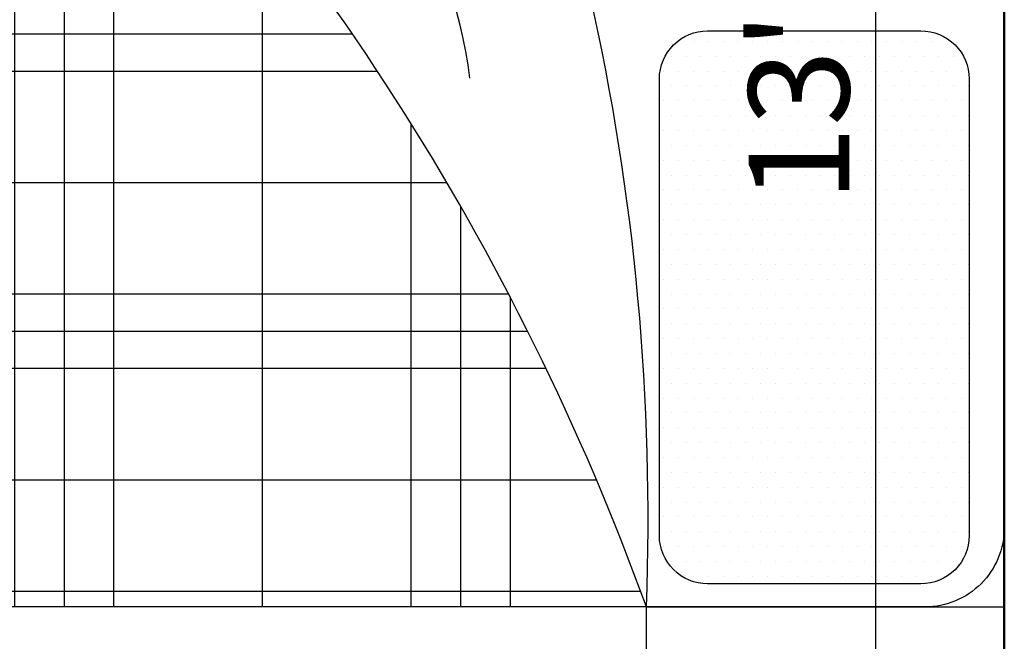
# Model space of a CAD drawing. Units: inches. Extents: x 3064 to 19385, y 846 to 15425.
# Tile 96 of 108: x 7612 to 7661, y 1032 to 1063. Entities that reach past the tile are written whole.
import ezdxf

# ---------------------------------------------------------------- set-up
doc = ezdxf.new("R2010")
doc.units = ezdxf.units.IN
for name, color, linetype, lineweight in [('A-ANNO-DIMS', 2, 'Continuous', 18), ('A-FLOR-FIXT', 9, 'Continuous', 18), ('A-WALL', 7, 'Continuous', 50)]:
    doc.layers.add(name, color=color, linetype=linetype, lineweight=lineweight)
doc.layers.add('BLOCK', color=6, linetype='Continuous')
doc.styles.get("Standard").update_dxf_attribs({"font": 'arial.ttf'})
doc.dimstyles.new('ISO-25', dxfattribs={"dimtxt": 9, "dimasz": 2.5, "dimexe": 1.25, "dimexo": 0.625, "dimtad": 1, "dimdec": 1, "dimlunit": 3, "dimtxsty": 'Standard', "dimcen": 2.5, "dimadec": 0, "dimazin": 0, "dimtfac": 1, "dimtdec": 1, "dimtmove": 0, "dimatfit": 3, "dimfxl": 1, "dimarcsym": 0})

# ---------------------------------------------------------------- blocks, each defined once
blk = doc.blocks.new('*D234')
at = {"layer": 'A-ANNO-DIMS', "color": 0, "lineweight": -2, "transparency": 16777216}
for p, q in [((7660.621, 1144.34), (7653.626, 1144.34)), ((7654.876, 984.84), (7654.876, 1141.84)), ((7660.621, 982.34), (7653.626, 982.34))]:
    blk.add_line(p, q, dxfattribs=at)
at = {"layer": 'A-ANNO-DIMS', "color": 0, "transparency": 16777216}
for points in [[(7654.459, 1141.84), (7655.292, 1141.84), (7654.876, 1144.34)], [(7654.459, 984.84), (7655.292, 984.84), (7654.876, 982.34)]]:
    blk.add_solid(points, dxfattribs=at)
at = {"layer": 'Defpoints', "color": 0, "transparency": 16777216}
for p in [(7654.876, 1144.34), (7661.246, 1144.34), (7661.246, 982.34)]:
    blk.add_point(p, dxfattribs=at)
at = {"layer": 'A-ANNO-DIMS', "color": 0, "transparency": 16777216, "insert": (7651.696, 1063.34), "char_height": 5, "attachment_point": 5, "rotation": 90}
blk.add_mtext('13\'-6"', dxfattribs=at)
blk = doc.blocks.new('*X5')
at = {"color": 0}
for p, q in [((276.598, 451.25), (280.51, 451.25)), ((275.455, 450.625), (280.51, 450.625)), ((274.411, 450), (280.51, 450)), ((265.51, 448.125), (267.634, 448.125)), ((271.723, 448.125), (280.51, 448.125)), ((265.51, 446.25), (268.465, 446.25)), ((269.519, 446.25), (280.51, 446.25)), ((265.51, 445.625), (268.531, 445.625)), ((268.866, 445.625), (280.51, 445.625)), ((265.51, 445), (280.51, 445)), ((265.51, 443.125), (280.51, 443.125)), ((265.51, 441.25), (280.51, 441.25)), ((265.51, 440.625), (280.51, 440.625)), ((265.634, 440), (280.386, 440))]:
    blk.add_line(p, q, dxfattribs=at)
blk = doc.blocks.new('*X6')
at = {"color": 0}
for p, q in [((280.312, 439.886), (280.312, 452.896)), ((278.906, 439.482), (278.906, 452.338)), ((277.5, 439.482), (277.5, 451.702)), ((277.031, 439.482), (277.031, 451.471)), ((276.562, 439.482), (276.562, 451.231)), ((275.156, 439.482), (275.156, 450.451)), ((273.75, 439.482), (273.75, 449.576)), ((273.281, 439.482), (273.281, 449.261))]:
    blk.add_line(p, q, dxfattribs=at)
blk = doc.blocks.new('*X7')
at = {"color": 0}
for p, q in [((273.9375, 457.03125), (273.9375, 457.03125)), ((274.3125, 457.03125), (274.3125, 457.03125)), ((274.6875, 457.03125), (274.6875, 457.03125)), ((275.0625, 457.03125), (275.0625, 457.03125)), ((275.4375, 457.03125), (275.4375, 457.03125)), ((275.8125, 457.03125), (275.8125, 457.03125)), ((276.1875, 457.03125), (276.1875, 457.03125)), ((276.5625, 457.03125), (276.5625, 457.03125)), ((276.9375, 457.03125), (276.9375, 457.03125)), ((277.3125, 457.03125), (277.3125, 457.03125)), ((277.6875, 457.03125), (277.6875, 457.03125)), ((278.0625, 457.03125), (278.0625, 457.03125)), ((278.4375, 457.03125), (278.4375, 457.03125)), ((278.8125, 457.03125), (278.8125, 457.03125)), ((279.1875, 457.03125), (279.1875, 457.03125)), ((279.5625, 457.03125), (279.5625, 457.03125)), ((273.75, 456.9375), (273.75, 456.9375)), ((274.125, 456.9375), (274.125, 456.9375)), ((274.5, 456.9375), (274.5, 456.9375)), ((274.875, 456.9375), (274.875, 456.9375)), ((275.25, 456.9375), (275.25, 456.9375)), ((275.625, 456.9375), (275.625, 456.9375)), ((276, 456.9375), (276, 456.9375)), ((276.375, 456.9375), (276.375, 456.9375)), ((276.75, 456.9375), (276.75, 456.9375)), ((277.125, 456.9375), (277.125, 456.9375)), ((277.5, 456.9375), (277.5, 456.9375)), ((277.875, 456.9375), (277.875, 456.9375)), ((278.25, 456.9375), (278.25, 456.9375)), ((278.625, 456.9375), (278.625, 456.9375)), ((279, 456.9375), (279, 456.9375)), ((279.375, 456.9375), (279.375, 456.9375)), ((279.75, 456.9375), (279.75, 456.9375)), ((273.5625, 456.84375), (273.5625, 456.84375)), ((273.9375, 456.84375), (273.9375, 456.84375)), ((274.3125, 456.84375), (274.3125, 456.84375)), ((274.6875, 456.84375), (274.6875, 456.84375)), ((275.0625, 456.84375), (275.0625, 456.84375)), ((275.4375, 456.84375), (275.4375, 456.84375)), ((275.8125, 456.84375), (275.8125, 456.84375)), ((276.1875, 456.84375), (276.1875, 456.84375)), ((276.5625, 456.84375), (276.5625, 456.84375)), ((276.9375, 456.84375), (276.9375, 456.84375)), ((277.3125, 456.84375), (277.3125, 456.84375)), ((277.6875, 456.84375), (277.6875, 456.84375)), ((278.0625, 456.84375), (278.0625, 456.84375)), ((278.4375, 456.84375), (278.4375, 456.84375)), ((278.8125, 456.84375), (278.8125, 456.84375)), ((279.1875, 456.84375), (279.1875, 456.84375)), ((279.5625, 456.84375), (279.5625, 456.84375)), ((279.9375, 456.84375), (279.9375, 456.84375)), ((273.375, 456.75), (273.375, 456.75)), ((273.5625, 456.65625), (273.5625, 456.65625)), ((273.75, 456.75), (273.75, 456.75)), ((273.9375, 456.65625), (273.9375, 456.65625)), ((274.125, 456.75), (274.125, 456.75)), ((274.3125, 456.65625), (274.3125, 456.65625)), ((274.5, 456.75), (274.5, 456.75)), ((274.6875, 456.65625), (274.6875, 456.65625)), ((274.875, 456.75), (274.875, 456.75)), ((275.0625, 456.65625), (275.0625, 456.65625)), ((275.25, 456.75), (275.25, 456.75)), ((275.4375, 456.65625), (275.4375, 456.65625)), ((275.625, 456.75), (275.625, 456.75)), ((275.8125, 456.65625), (275.8125, 456.65625)), ((276, 456.75), (276, 456.75)), ((276.1875, 456.65625), (276.1875, 456.65625)), ((276.375, 456.75), (276.375, 456.75)), ((276.5625, 456.65625), (276.5625, 456.65625)), ((276.75, 456.75), (276.75, 456.75)), ((276.9375, 456.65625), (276.9375, 456.65625)), ((277.125, 456.75), (277.125, 456.75)), ((277.3125, 456.65625), (277.3125, 456.65625)), ((277.5, 456.75), (277.5, 456.75)), ((277.6875, 456.65625), (277.6875, 456.65625)), ((277.875, 456.75), (277.875, 456.75)), ((278.0625, 456.65625), (278.0625, 456.65625)), ((278.25, 456.75), (278.25, 456.75)), ((278.4375, 456.65625), (278.4375, 456.65625)), ((278.625, 456.75), (278.625, 456.75)), ((278.8125, 456.65625), (278.8125, 456.65625)), ((279, 456.75), (279, 456.75)), ((279.1875, 456.65625), (279.1875, 456.65625)), ((279.375, 456.75), (279.375, 456.75)), ((279.5625, 456.65625), (279.5625, 456.65625)), ((279.75, 456.75), (279.75, 456.75)), ((279.9375, 456.65625), (279.9375, 456.65625)), ((280.125, 456.75), (280.125, 456.75)), ((273.375, 456.5625), (273.375, 456.5625)), ((273.75, 456.5625), (273.75, 456.5625)), ((274.125, 456.5625), (274.125, 456.5625)), ((274.5, 456.5625), (274.5, 456.5625)), ((274.875, 456.5625), (274.875, 456.5625)), ((275.25, 456.5625), (275.25, 456.5625)), ((275.625, 456.5625), (275.625, 456.5625)), ((276, 456.5625), (276, 456.5625)), ((276.375, 456.5625), (276.375, 456.5625)), ((276.75, 456.5625), (276.75, 456.5625)), ((277.125, 456.5625), (277.125, 456.5625)), ((277.5, 456.5625), (277.5, 456.5625)), ((277.875, 456.5625), (277.875, 456.5625)), ((278.25, 456.5625), (278.25, 456.5625)), ((278.625, 456.5625), (278.625, 456.5625)), ((279, 456.5625), (279, 456.5625)), ((279.375, 456.5625), (279.375, 456.5625)), ((279.75, 456.5625), (279.75, 456.5625)), ((280.125, 456.5625), (280.125, 456.5625)), ((273.5625, 456.46875), (273.5625, 456.46875)), ((273.9375, 456.46875), (273.9375, 456.46875)), ((274.3125, 456.46875), (274.3125, 456.46875)), ((274.6875, 456.46875), (274.6875, 456.46875)), ((275.0625, 456.46875), (275.0625, 456.46875)), ((275.4375, 456.46875), (275.4375, 456.46875)), ((275.8125, 456.46875), (275.8125, 456.46875)), ((276.1875, 456.46875), (276.1875, 456.46875)), ((276.5625, 456.46875), (276.5625, 456.46875)), ((276.9375, 456.46875), (276.9375, 456.46875)), ((277.3125, 456.46875), (277.3125, 456.46875)), ((277.6875, 456.46875), (277.6875, 456.46875)), ((278.0625, 456.46875), (278.0625, 456.46875)), ((278.4375, 456.46875), (278.4375, 456.46875)), ((278.8125, 456.46875), (278.8125, 456.46875)), ((279.1875, 456.46875), (279.1875, 456.46875)), ((279.5625, 456.46875), (279.5625, 456.46875)), ((279.9375, 456.46875), (279.9375, 456.46875)), ((273.375, 456.375), (273.375, 456.375)), ((273.75, 456.375), (273.75, 456.375)), ((274.125, 456.375), (274.125, 456.375)), ((274.5, 456.375), (274.5, 456.375)), ((274.875, 456.375), (274.875, 456.375)), ((275.25, 456.375), (275.25, 456.375)), ((275.625, 456.375), (275.625, 456.375)), ((276, 456.375), (276, 456.375)), ((276.375, 456.375), (276.375, 456.375)), ((276.75, 456.375), (276.75, 456.375)), ((277.125, 456.375), (277.125, 456.375)), ((277.5, 456.375), (277.5, 456.375)), ((277.875, 456.375), (277.875, 456.375)), ((278.25, 456.375), (278.25, 456.375)), ((278.625, 456.375), (278.625, 456.375)), ((279, 456.375), (279, 456.375)), ((279.375, 456.375), (279.375, 456.375)), ((279.75, 456.375), (279.75, 456.375)), ((280.125, 456.375), (280.125, 456.375)), ((273.375, 456.1875), (273.375, 456.1875)), ((273.5625, 456.28125), (273.5625, 456.28125)), ((273.75, 456.1875), (273.75, 456.1875)), ((273.9375, 456.28125), (273.9375, 456.28125)), ((274.125, 456.1875), (274.125, 456.1875)), ((274.3125, 456.28125), (274.3125, 456.28125)), ((274.5, 456.1875), (274.5, 456.1875)), ((274.6875, 456.28125), (274.6875, 456.28125)), ((274.875, 456.1875), (274.875, 456.1875)), ((275.0625, 456.28125), (275.0625, 456.28125)), ((275.25, 456.1875), (275.25, 456.1875)), ((275.4375, 456.28125), (275.4375, 456.28125)), ((275.625, 456.1875), (275.625, 456.1875)), ((275.8125, 456.28125), (275.8125, 456.28125)), ((276, 456.1875), (276, 456.1875)), ((276.1875, 456.28125), (276.1875, 456.28125)), ((276.375, 456.1875), (276.375, 456.1875)), ((276.5625, 456.28125), (276.5625, 456.28125)), ((276.75, 456.1875), (276.75, 456.1875)), ((276.9375, 456.28125), (276.9375, 456.28125)), ((277.125, 456.1875), (277.125, 456.1875)), ((277.3125, 456.28125), (277.3125, 456.28125)), ((277.5, 456.1875), (277.5, 456.1875)), ((277.6875, 456.28125), (277.6875, 456.28125)), ((277.875, 456.1875), (277.875, 456.1875)), ((278.0625, 456.28125), (278.0625, 456.28125)), ((278.25, 456.1875), (278.25, 456.1875)), ((278.4375, 456.28125), (278.4375, 456.28125)), ((278.625, 456.1875), (278.625, 456.1875)), ((278.8125, 456.28125), (278.8125, 456.28125)), ((279, 456.1875), (279, 456.1875)), ((279.1875, 456.28125), (279.1875, 456.28125)), ((279.375, 456.1875), (279.375, 456.1875)), ((279.5625, 456.28125), (279.5625, 456.28125)), ((279.75, 456.1875), (279.75, 456.1875)), ((279.9375, 456.28125), (279.9375, 456.28125)), ((280.125, 456.1875), (280.125, 456.1875)), ((273.5625, 456.09375), (273.5625, 456.09375)), ((273.9375, 456.09375), (273.9375, 456.09375)), ((274.3125, 456.09375), (274.3125, 456.09375)), ((274.6875, 456.09375), (274.6875, 456.09375)), ((275.0625, 456.09375), (275.0625, 456.09375)), ((275.4375, 456.09375), (275.4375, 456.09375)), ((275.8125, 456.09375), (275.8125, 456.09375)), ((276.1875, 456.09375), (276.1875, 456.09375)), ((276.5625, 456.09375), (276.5625, 456.09375)), ((276.9375, 456.09375), (276.9375, 456.09375)), ((277.3125, 456.09375), (277.3125, 456.09375)), ((277.6875, 456.09375), (277.6875, 456.09375)), ((278.0625, 456.09375), (278.0625, 456.09375)), ((278.4375, 456.09375), (278.4375, 456.09375)), ((278.8125, 456.09375), (278.8125, 456.09375)), ((279.1875, 456.09375), (279.1875, 456.09375)), ((279.5625, 456.09375), (279.5625, 456.09375)), ((279.9375, 456.09375), (279.9375, 456.09375)), ((273.375, 456), (273.375, 456)), ((273.75, 456), (273.75, 456)), ((274.125, 456), (274.125, 456)), ((274.5, 456), (274.5, 456)), ((274.875, 456), (274.875, 456)), ((275.25, 456), (275.25, 456)), ((275.625, 456), (275.625, 456)), ((276, 456), (276, 456)), ((276.375, 456), (276.375, 456)), ((276.75, 456), (276.75, 456)), ((277.125, 456), (277.125, 456)), ((277.5, 456), (277.5, 456)), ((277.875, 456), (277.875, 456)), ((278.25, 456), (278.25, 456)), ((278.625, 456), (278.625, 456)), ((279, 456), (279, 456)), ((279.375, 456), (279.375, 456)), ((279.75, 456), (279.75, 456)), ((280.125, 456), (280.125, 456)), ((273.375, 455.8125), (273.375, 455.8125)), ((273.5625, 455.90625), (273.5625, 455.90625)), ((273.75, 455.8125), (273.75, 455.8125)), ((273.9375, 455.90625), (273.9375, 455.90625)), ((274.125, 455.8125), (274.125, 455.8125)), ((274.3125, 455.90625), (274.3125, 455.90625)), ((274.5, 455.8125), (274.5, 455.8125)), ((274.6875, 455.90625), (274.6875, 455.90625)), ((274.875, 455.8125), (274.875, 455.8125)), ((275.0625, 455.90625), (275.0625, 455.90625)), ((275.25, 455.8125), (275.25, 455.8125)), ((275.4375, 455.90625), (275.4375, 455.90625)), ((275.625, 455.8125), (275.625, 455.8125)), ((275.8125, 455.90625), (275.8125, 455.90625)), ((276, 455.8125), (276, 455.8125)), ((276.1875, 455.90625), (276.1875, 455.90625)), ((276.375, 455.8125), (276.375, 455.8125)), ((276.5625, 455.90625), (276.5625, 455.90625)), ((276.75, 455.8125), (276.75, 455.8125)), ((276.9375, 455.90625), (276.9375, 455.90625)), ((277.125, 455.8125), (277.125, 455.8125)), ((277.3125, 455.90625), (277.3125, 455.90625)), ((277.5, 455.8125), (277.5, 455.8125)), ((277.6875, 455.90625), (277.6875, 455.90625)), ((277.875, 455.8125), (277.875, 455.8125)), ((278.0625, 455.90625), (278.0625, 455.90625)), ((278.25, 455.8125), (278.25, 455.8125)), ((278.4375, 455.90625), (278.4375, 455.90625)), ((278.625, 455.8125), (278.625, 455.8125)), ((278.8125, 455.90625), (278.8125, 455.90625)), ((279, 455.8125), (279, 455.8125)), ((279.1875, 455.90625), (279.1875, 455.90625)), ((279.375, 455.8125), (279.375, 455.8125)), ((279.5625, 455.90625), (279.5625, 455.90625)), ((279.75, 455.8125), (279.75, 455.8125)), ((279.9375, 455.90625), (279.9375, 455.90625)), ((280.125, 455.8125), (280.125, 455.8125)), ((273.5625, 455.71875), (273.5625, 455.71875)), ((273.9375, 455.71875), (273.9375, 455.71875)), ((274.3125, 455.71875), (274.3125, 455.71875)), ((274.6875, 455.71875), (274.6875, 455.71875)), ((275.0625, 455.71875), (275.0625, 455.71875)), ((275.4375, 455.71875), (275.4375, 455.71875)), ((275.8125, 455.71875), (275.8125, 455.71875)), ((276.1875, 455.71875), (276.1875, 455.71875)), ((276.5625, 455.71875), (276.5625, 455.71875)), ((276.9375, 455.71875), (276.9375, 455.71875)), ((277.3125, 455.71875), (277.3125, 455.71875)), ((277.6875, 455.71875), (277.6875, 455.71875)), ((278.0625, 455.71875), (278.0625, 455.71875)), ((278.4375, 455.71875), (278.4375, 455.71875)), ((278.8125, 455.71875), (278.8125, 455.71875)), ((279.1875, 455.71875), (279.1875, 455.71875)), ((279.5625, 455.71875), (279.5625, 455.71875)), ((279.9375, 455.71875), (279.9375, 455.71875)), ((273.375, 455.625), (273.375, 455.625)), ((273.75, 455.625), (273.75, 455.625)), ((274.125, 455.625), (274.125, 455.625)), ((274.5, 455.625), (274.5, 455.625)), ((274.875, 455.625), (274.875, 455.625)), ((275.25, 455.625), (275.25, 455.625)), ((275.625, 455.625), (275.625, 455.625)), ((276, 455.625), (276, 455.625)), ((276.375, 455.625), (276.375, 455.625)), ((276.75, 455.625), (276.75, 455.625)), ((277.125, 455.625), (277.125, 455.625)), ((277.5, 455.625), (277.5, 455.625)), ((277.875, 455.625), (277.875, 455.625)), ((278.25, 455.625), (278.25, 455.625)), ((278.625, 455.625), (278.625, 455.625)), ((279, 455.625), (279, 455.625)), ((279.375, 455.625), (279.375, 455.625)), ((279.75, 455.625), (279.75, 455.625)), ((280.125, 455.625), (280.125, 455.625)), ((273.375, 455.4375), (273.375, 455.4375)), ((273.5625, 455.53125), (273.5625, 455.53125)), ((273.75, 455.4375), (273.75, 455.4375)), ((273.9375, 455.53125), (273.9375, 455.53125)), ((274.125, 455.4375), (274.125, 455.4375)), ((274.3125, 455.53125), (274.3125, 455.53125)), ((274.5, 455.4375), (274.5, 455.4375)), ((274.6875, 455.53125), (274.6875, 455.53125)), ((274.875, 455.4375), (274.875, 455.4375)), ((275.0625, 455.53125), (275.0625, 455.53125)), ((275.25, 455.4375), (275.25, 455.4375)), ((275.4375, 455.53125), (275.4375, 455.53125)), ((275.625, 455.4375), (275.625, 455.4375)), ((275.8125, 455.53125), (275.8125, 455.53125)), ((276, 455.4375), (276, 455.4375)), ((276.1875, 455.53125), (276.1875, 455.53125)), ((276.375, 455.4375), (276.375, 455.4375)), ((276.5625, 455.53125), (276.5625, 455.53125)), ((276.75, 455.4375), (276.75, 455.4375)), ((276.9375, 455.53125), (276.9375, 455.53125)), ((277.125, 455.4375), (277.125, 455.4375)), ((277.3125, 455.53125), (277.3125, 455.53125)), ((277.5, 455.4375), (277.5, 455.4375)), ((277.6875, 455.53125), (277.6875, 455.53125)), ((277.875, 455.4375), (277.875, 455.4375)), ((278.0625, 455.53125), (278.0625, 455.53125)), ((278.25, 455.4375), (278.25, 455.4375)), ((278.4375, 455.53125), (278.4375, 455.53125)), ((278.625, 455.4375), (278.625, 455.4375)), ((278.8125, 455.53125), (278.8125, 455.53125)), ((279, 455.4375), (279, 455.4375)), ((279.1875, 455.53125), (279.1875, 455.53125)), ((279.375, 455.4375), (279.375, 455.4375)), ((279.5625, 455.53125), (279.5625, 455.53125)), ((279.75, 455.4375), (279.75, 455.4375)), ((279.9375, 455.53125), (279.9375, 455.53125)), ((280.125, 455.4375), (280.125, 455.4375)), ((273.5625, 455.34375), (273.5625, 455.34375)), ((273.9375, 455.34375), (273.9375, 455.34375)), ((274.3125, 455.34375), (274.3125, 455.34375)), ((274.6875, 455.34375), (274.6875, 455.34375)), ((275.0625, 455.34375), (275.0625, 455.34375)), ((275.4375, 455.34375), (275.4375, 455.34375)), ((275.8125, 455.34375), (275.8125, 455.34375)), ((276.1875, 455.34375), (276.1875, 455.34375)), ((276.5625, 455.34375), (276.5625, 455.34375)), ((276.9375, 455.34375), (276.9375, 455.34375)), ((277.3125, 455.34375), (277.3125, 455.34375)), ((277.6875, 455.34375), (277.6875, 455.34375)), ((278.0625, 455.34375), (278.0625, 455.34375)), ((278.4375, 455.34375), (278.4375, 455.34375)), ((278.8125, 455.34375), (278.8125, 455.34375)), ((279.1875, 455.34375), (279.1875, 455.34375)), ((279.5625, 455.34375), (279.5625, 455.34375)), ((279.9375, 455.34375), (279.9375, 455.34375)), ((273.375, 455.25), (273.375, 455.25)), ((273.75, 455.25), (273.75, 455.25)), ((274.125, 455.25), (274.125, 455.25)), ((274.5, 455.25), (274.5, 455.25)), ((274.875, 455.25), (274.875, 455.25)), ((275.25, 455.25), (275.25, 455.25)), ((275.625, 455.25), (275.625, 455.25)), ((276, 455.25), (276, 455.25)), ((276.375, 455.25), (276.375, 455.25)), ((276.75, 455.25), (276.75, 455.25)), ((277.125, 455.25), (277.125, 455.25)), ((277.5, 455.25), (277.5, 455.25)), ((277.875, 455.25), (277.875, 455.25)), ((278.25, 455.25), (278.25, 455.25)), ((278.625, 455.25), (278.625, 455.25)), ((279, 455.25), (279, 455.25)), ((279.375, 455.25), (279.375, 455.25)), ((279.75, 455.25), (279.75, 455.25)), ((280.125, 455.25), (280.125, 455.25)), ((273.375, 455.0625), (273.375, 455.0625)), ((273.5625, 455.15625), (273.5625, 455.15625)), ((273.75, 455.0625), (273.75, 455.0625)), ((273.9375, 455.15625), (273.9375, 455.15625)), ((274.125, 455.0625), (274.125, 455.0625)), ((274.3125, 455.15625), (274.3125, 455.15625)), ((274.5, 455.0625), (274.5, 455.0625)), ((274.6875, 455.15625), (274.6875, 455.15625)), ((274.875, 455.0625), (274.875, 455.0625)), ((275.0625, 455.15625), (275.0625, 455.15625)), ((275.25, 455.0625), (275.25, 455.0625)), ((275.4375, 455.15625), (275.4375, 455.15625)), ((275.625, 455.0625), (275.625, 455.0625)), ((275.8125, 455.15625), (275.8125, 455.15625)), ((276, 455.0625), (276, 455.0625)), ((276.1875, 455.15625), (276.1875, 455.15625)), ((276.375, 455.0625), (276.375, 455.0625)), ((276.5625, 455.15625), (276.5625, 455.15625)), ((276.75, 455.0625), (276.75, 455.0625)), ((276.9375, 455.15625), (276.9375, 455.15625)), ((277.125, 455.0625), (277.125, 455.0625)), ((277.3125, 455.15625), (277.3125, 455.15625)), ((277.5, 455.0625), (277.5, 455.0625)), ((277.6875, 455.15625), (277.6875, 455.15625)), ((277.875, 455.0625), (277.875, 455.0625)), ((278.0625, 455.15625), (278.0625, 455.15625)), ((278.25, 455.0625), (278.25, 455.0625)), ((278.4375, 455.15625), (278.4375, 455.15625)), ((278.625, 455.0625), (278.625, 455.0625)), ((278.8125, 455.15625), (278.8125, 455.15625)), ((279, 455.0625), (279, 455.0625)), ((279.1875, 455.15625), (279.1875, 455.15625)), ((279.375, 455.0625), (279.375, 455.0625)), ((279.5625, 455.15625), (279.5625, 455.15625)), ((279.75, 455.0625), (279.75, 455.0625)), ((279.9375, 455.15625), (279.9375, 455.15625)), ((280.125, 455.0625), (280.125, 455.0625)), ((273.5625, 454.96875), (273.5625, 454.96875)), ((273.9375, 454.96875), (273.9375, 454.96875)), ((274.3125, 454.96875), (274.3125, 454.96875)), ((274.6875, 454.96875), (274.6875, 454.96875)), ((275.0625, 454.96875), (275.0625, 454.96875)), ((275.4375, 454.96875), (275.4375, 454.96875)), ((275.8125, 454.96875), (275.8125, 454.96875)), ((276.1875, 454.96875), (276.1875, 454.96875)), ((276.5625, 454.96875), (276.5625, 454.96875)), ((276.9375, 454.96875), (276.9375, 454.96875)), ((277.3125, 454.96875), (277.3125, 454.96875)), ((277.6875, 454.96875), (277.6875, 454.96875)), ((278.0625, 454.96875), (278.0625, 454.96875)), ((278.4375, 454.96875), (278.4375, 454.96875)), ((278.8125, 454.96875), (278.8125, 454.96875)), ((279.1875, 454.96875), (279.1875, 454.96875)), ((279.5625, 454.96875), (279.5625, 454.96875)), ((279.9375, 454.96875), (279.9375, 454.96875)), ((273.375, 454.875), (273.375, 454.875)), ((273.75, 454.875), (273.75, 454.875)), ((274.125, 454.875), (274.125, 454.875)), ((274.5, 454.875), (274.5, 454.875)), ((274.875, 454.875), (274.875, 454.875)), ((275.25, 454.875), (275.25, 454.875)), ((275.625, 454.875), (275.625, 454.875)), ((276, 454.875), (276, 454.875)), ((276.375, 454.875), (276.375, 454.875)), ((276.75, 454.875), (276.75, 454.875)), ((277.125, 454.875), (277.125, 454.875)), ((277.5, 454.875), (277.5, 454.875)), ((277.875, 454.875), (277.875, 454.875)), ((278.25, 454.875), (278.25, 454.875)), ((278.625, 454.875), (278.625, 454.875)), ((279, 454.875), (279, 454.875)), ((279.375, 454.875), (279.375, 454.875)), ((279.75, 454.875), (279.75, 454.875)), ((280.125, 454.875), (280.125, 454.875)), ((273.375, 454.6875), (273.375, 454.6875)), ((273.5625, 454.78125), (273.5625, 454.78125)), ((273.75, 454.6875), (273.75, 454.6875)), ((273.9375, 454.78125), (273.9375, 454.78125)), ((274.125, 454.6875), (274.125, 454.6875)), ((274.3125, 454.78125), (274.3125, 454.78125)), ((274.5, 454.6875), (274.5, 454.6875)), ((274.6875, 454.78125), (274.6875, 454.78125)), ((274.875, 454.6875), (274.875, 454.6875)), ((275.0625, 454.78125), (275.0625, 454.78125)), ((275.25, 454.6875), (275.25, 454.6875)), ((275.4375, 454.78125), (275.4375, 454.78125)), ((275.625, 454.6875), (275.625, 454.6875)), ((275.8125, 454.78125), (275.8125, 454.78125)), ((276, 454.6875), (276, 454.6875)), ((276.1875, 454.78125), (276.1875, 454.78125)), ((276.375, 454.6875), (276.375, 454.6875)), ((276.5625, 454.78125), (276.5625, 454.78125)), ((276.75, 454.6875), (276.75, 454.6875)), ((276.9375, 454.78125), (276.9375, 454.78125)), ((277.125, 454.6875), (277.125, 454.6875)), ((277.3125, 454.78125), (277.3125, 454.78125)), ((277.5, 454.6875), (277.5, 454.6875)), ((277.6875, 454.78125), (277.6875, 454.78125)), ((277.875, 454.6875), (277.875, 454.6875)), ((278.0625, 454.78125), (278.0625, 454.78125)), ((278.25, 454.6875), (278.25, 454.6875)), ((278.4375, 454.78125), (278.4375, 454.78125)), ((278.625, 454.6875), (278.625, 454.6875)), ((278.8125, 454.78125), (278.8125, 454.78125)), ((279, 454.6875), (279, 454.6875)), ((279.1875, 454.78125), (279.1875, 454.78125)), ((279.375, 454.6875), (279.375, 454.6875)), ((279.5625, 454.78125), (279.5625, 454.78125)), ((279.75, 454.6875), (279.75, 454.6875)), ((279.9375, 454.78125), (279.9375, 454.78125)), ((280.125, 454.6875), (280.125, 454.6875)), ((273.5625, 454.59375), (273.5625, 454.59375)), ((273.9375, 454.59375), (273.9375, 454.59375)), ((274.3125, 454.59375), (274.3125, 454.59375)), ((274.6875, 454.59375), (274.6875, 454.59375)), ((275.0625, 454.59375), (275.0625, 454.59375)), ((275.4375, 454.59375), (275.4375, 454.59375)), ((275.8125, 454.59375), (275.8125, 454.59375)), ((276.1875, 454.59375), (276.1875, 454.59375)), ((276.5625, 454.59375), (276.5625, 454.59375)), ((276.9375, 454.59375), (276.9375, 454.59375)), ((277.3125, 454.59375), (277.3125, 454.59375)), ((277.6875, 454.59375), (277.6875, 454.59375)), ((278.0625, 454.59375), (278.0625, 454.59375)), ((278.4375, 454.59375), (278.4375, 454.59375)), ((278.8125, 454.59375), (278.8125, 454.59375)), ((279.1875, 454.59375), (279.1875, 454.59375)), ((279.5625, 454.59375), (279.5625, 454.59375)), ((279.9375, 454.59375), (279.9375, 454.59375)), ((273.375, 454.5), (273.375, 454.5)), ((273.75, 454.5), (273.75, 454.5)), ((274.125, 454.5), (274.125, 454.5)), ((274.5, 454.5), (274.5, 454.5)), ((274.875, 454.5), (274.875, 454.5)), ((275.25, 454.5), (275.25, 454.5)), ((275.625, 454.5), (275.625, 454.5)), ((276, 454.5), (276, 454.5)), ((276.375, 454.5), (276.375, 454.5)), ((276.75, 454.5), (276.75, 454.5)), ((277.125, 454.5), (277.125, 454.5)), ((277.5, 454.5), (277.5, 454.5)), ((277.875, 454.5), (277.875, 454.5)), ((278.25, 454.5), (278.25, 454.5)), ((278.625, 454.5), (278.625, 454.5)), ((279, 454.5), (279, 454.5)), ((279.375, 454.5), (279.375, 454.5)), ((279.75, 454.5), (279.75, 454.5)), ((280.125, 454.5), (280.125, 454.5)), ((273.375, 454.3125), (273.375, 454.3125)), ((273.5625, 454.40625), (273.5625, 454.40625)), ((273.75, 454.3125), (273.75, 454.3125)), ((273.9375, 454.40625), (273.9375, 454.40625)), ((274.125, 454.3125), (274.125, 454.3125)), ((274.3125, 454.40625), (274.3125, 454.40625)), ((274.5, 454.3125), (274.5, 454.3125)), ((274.6875, 454.40625), (274.6875, 454.40625)), ((274.875, 454.3125), (274.875, 454.3125)), ((275.0625, 454.40625), (275.0625, 454.40625)), ((275.25, 454.3125), (275.25, 454.3125)), ((275.4375, 454.40625), (275.4375, 454.40625)), ((275.625, 454.3125), (275.625, 454.3125)), ((275.8125, 454.40625), (275.8125, 454.40625)), ((276, 454.3125), (276, 454.3125)), ((276.1875, 454.40625), (276.1875, 454.40625)), ((276.375, 454.3125), (276.375, 454.3125)), ((276.5625, 454.40625), (276.5625, 454.40625)), ((276.75, 454.3125), (276.75, 454.3125)), ((276.9375, 454.40625), (276.9375, 454.40625)), ((277.125, 454.3125), (277.125, 454.3125)), ((277.3125, 454.40625), (277.3125, 454.40625)), ((277.5, 454.3125), (277.5, 454.3125)), ((277.6875, 454.40625), (277.6875, 454.40625)), ((277.875, 454.3125), (277.875, 454.3125)), ((278.0625, 454.40625), (278.0625, 454.40625)), ((278.25, 454.3125), (278.25, 454.3125)), ((278.4375, 454.40625), (278.4375, 454.40625)), ((278.625, 454.3125), (278.625, 454.3125)), ((278.8125, 454.40625), (278.8125, 454.40625)), ((279, 454.3125), (279, 454.3125)), ((279.1875, 454.40625), (279.1875, 454.40625)), ((279.375, 454.3125), (279.375, 454.3125)), ((279.5625, 454.40625), (279.5625, 454.40625)), ((279.75, 454.3125), (279.75, 454.3125)), ((279.9375, 454.40625), (279.9375, 454.40625)), ((280.125, 454.3125), (280.125, 454.3125)), ((273.5625, 454.21875), (273.5625, 454.21875)), ((273.9375, 454.21875), (273.9375, 454.21875)), ((274.3125, 454.21875), (274.3125, 454.21875)), ((274.6875, 454.21875), (274.6875, 454.21875)), ((275.0625, 454.21875), (275.0625, 454.21875)), ((275.4375, 454.21875), (275.4375, 454.21875)), ((275.8125, 454.21875), (275.8125, 454.21875)), ((276.1875, 454.21875), (276.1875, 454.21875)), ((276.5625, 454.21875), (276.5625, 454.21875)), ((276.9375, 454.21875), (276.9375, 454.21875)), ((277.3125, 454.21875), (277.3125, 454.21875)), ((277.6875, 454.21875), (277.6875, 454.21875)), ((278.0625, 454.21875), (278.0625, 454.21875)), ((278.4375, 454.21875), (278.4375, 454.21875)), ((278.8125, 454.21875), (278.8125, 454.21875)), ((279.1875, 454.21875), (279.1875, 454.21875)), ((279.5625, 454.21875), (279.5625, 454.21875)), ((279.9375, 454.21875), (279.9375, 454.21875)), ((273.375, 454.125), (273.375, 454.125)), ((273.75, 454.125), (273.75, 454.125)), ((274.125, 454.125), (274.125, 454.125)), ((274.5, 454.125), (274.5, 454.125)), ((274.875, 454.125), (274.875, 454.125)), ((275.25, 454.125), (275.25, 454.125)), ((275.625, 454.125), (275.625, 454.125)), ((276, 454.125), (276, 454.125)), ((276.375, 454.125), (276.375, 454.125)), ((276.75, 454.125), (276.75, 454.125)), ((277.125, 454.125), (277.125, 454.125)), ((277.5, 454.125), (277.5, 454.125)), ((277.875, 454.125), (277.875, 454.125)), ((278.25, 454.125), (278.25, 454.125)), ((278.625, 454.125), (278.625, 454.125)), ((279, 454.125), (279, 454.125)), ((279.375, 454.125), (279.375, 454.125)), ((279.75, 454.125), (279.75, 454.125)), ((280.125, 454.125), (280.125, 454.125)), ((273.375, 453.9375), (273.375, 453.9375)), ((273.5625, 454.03125), (273.5625, 454.03125)), ((273.75, 453.9375), (273.75, 453.9375)), ((273.9375, 454.03125), (273.9375, 454.03125)), ((274.125, 453.9375), (274.125, 453.9375)), ((274.3125, 454.03125), (274.3125, 454.03125)), ((274.5, 453.9375), (274.5, 453.9375)), ((274.6875, 454.03125), (274.6875, 454.03125)), ((274.875, 453.9375), (274.875, 453.9375)), ((275.0625, 454.03125), (275.0625, 454.03125)), ((275.25, 453.9375), (275.25, 453.9375)), ((275.4375, 454.03125), (275.4375, 454.03125)), ((275.625, 453.9375), (275.625, 453.9375)), ((275.8125, 454.03125), (275.8125, 454.03125)), ((276, 453.9375), (276, 453.9375)), ((276.1875, 454.03125), (276.1875, 454.03125)), ((276.375, 453.9375), (276.375, 453.9375)), ((276.5625, 454.03125), (276.5625, 454.03125)), ((276.75, 453.9375), (276.75, 453.9375)), ((276.9375, 454.03125), (276.9375, 454.03125)), ((277.125, 453.9375), (277.125, 453.9375)), ((277.3125, 454.03125), (277.3125, 454.03125)), ((277.5, 453.9375), (277.5, 453.9375)), ((277.6875, 454.03125), (277.6875, 454.03125)), ((277.875, 453.9375), (277.875, 453.9375)), ((278.0625, 454.03125), (278.0625, 454.03125)), ((278.25, 453.9375), (278.25, 453.9375)), ((278.4375, 454.03125), (278.4375, 454.03125)), ((278.625, 453.9375), (278.625, 453.9375)), ((278.8125, 454.03125), (278.8125, 454.03125)), ((279, 453.9375), (279, 453.9375)), ((279.1875, 454.03125), (279.1875, 454.03125)), ((279.375, 453.9375), (279.375, 453.9375)), ((279.5625, 454.03125), (279.5625, 454.03125)), ((279.75, 453.9375), (279.75, 453.9375)), ((279.9375, 454.03125), (279.9375, 454.03125)), ((280.125, 453.9375), (280.125, 453.9375)), ((273.5625, 453.84375), (273.5625, 453.84375)), ((273.9375, 453.84375), (273.9375, 453.84375)), ((274.3125, 453.84375), (274.3125, 453.84375)), ((274.6875, 453.84375), (274.6875, 453.84375)), ((275.0625, 453.84375), (275.0625, 453.84375)), ((275.4375, 453.84375), (275.4375, 453.84375)), ((275.8125, 453.84375), (275.8125, 453.84375)), ((276.1875, 453.84375), (276.1875, 453.84375)), ((276.5625, 453.84375), (276.5625, 453.84375)), ((276.9375, 453.84375), (276.9375, 453.84375)), ((277.3125, 453.84375), (277.3125, 453.84375)), ((277.6875, 453.84375), (277.6875, 453.84375)), ((278.0625, 453.84375), (278.0625, 453.84375)), ((278.4375, 453.84375), (278.4375, 453.84375)), ((278.8125, 453.84375), (278.8125, 453.84375)), ((279.1875, 453.84375), (279.1875, 453.84375)), ((279.5625, 453.84375), (279.5625, 453.84375)), ((279.9375, 453.84375), (279.9375, 453.84375)), ((273.375, 453.75), (273.375, 453.75)), ((273.75, 453.75), (273.75, 453.75)), ((274.125, 453.75), (274.125, 453.75)), ((274.5, 453.75), (274.5, 453.75)), ((274.875, 453.75), (274.875, 453.75)), ((275.25, 453.75), (275.25, 453.75)), ((275.625, 453.75), (275.625, 453.75)), ((276, 453.75), (276, 453.75)), ((276.375, 453.75), (276.375, 453.75)), ((276.75, 453.75), (276.75, 453.75)), ((277.125, 453.75), (277.125, 453.75)), ((277.5, 453.75), (277.5, 453.75)), ((277.875, 453.75), (277.875, 453.75)), ((278.25, 453.75), (278.25, 453.75)), ((278.625, 453.75), (278.625, 453.75)), ((279, 453.75), (279, 453.75)), ((279.375, 453.75), (279.375, 453.75)), ((279.75, 453.75), (279.75, 453.75)), ((280.125, 453.75), (280.125, 453.75)), ((273.375, 453.5625), (273.375, 453.5625)), ((273.5625, 453.65625), (273.5625, 453.65625)), ((273.75, 453.5625), (273.75, 453.5625)), ((273.9375, 453.65625), (273.9375, 453.65625)), ((274.125, 453.5625), (274.125, 453.5625)), ((274.3125, 453.65625), (274.3125, 453.65625)), ((274.5, 453.5625), (274.5, 453.5625)), ((274.6875, 453.65625), (274.6875, 453.65625)), ((274.875, 453.5625), (274.875, 453.5625)), ((275.0625, 453.65625), (275.0625, 453.65625)), ((275.25, 453.5625), (275.25, 453.5625)), ((275.4375, 453.65625), (275.4375, 453.65625)), ((275.625, 453.5625), (275.625, 453.5625)), ((275.8125, 453.65625), (275.8125, 453.65625)), ((276, 453.5625), (276, 453.5625)), ((276.1875, 453.65625), (276.1875, 453.65625)), ((276.375, 453.5625), (276.375, 453.5625)), ((276.5625, 453.65625), (276.5625, 453.65625)), ((276.75, 453.5625), (276.75, 453.5625)), ((276.9375, 453.65625), (276.9375, 453.65625)), ((277.125, 453.5625), (277.125, 453.5625)), ((277.3125, 453.65625), (277.3125, 453.65625)), ((277.5, 453.5625), (277.5, 453.5625)), ((277.6875, 453.65625), (277.6875, 453.65625)), ((277.875, 453.5625), (277.875, 453.5625)), ((278.0625, 453.65625), (278.0625, 453.65625)), ((278.25, 453.5625), (278.25, 453.5625)), ((278.4375, 453.65625), (278.4375, 453.65625)), ((278.625, 453.5625), (278.625, 453.5625)), ((278.8125, 453.65625), (278.8125, 453.65625)), ((279, 453.5625), (279, 453.5625)), ((279.1875, 453.65625), (279.1875, 453.65625)), ((279.375, 453.5625), (279.375, 453.5625)), ((279.5625, 453.65625), (279.5625, 453.65625)), ((279.75, 453.5625), (279.75, 453.5625)), ((279.9375, 453.65625), (279.9375, 453.65625)), ((280.125, 453.5625), (280.125, 453.5625)), ((273.5625, 453.46875), (273.5625, 453.46875)), ((273.9375, 453.46875), (273.9375, 453.46875)), ((274.3125, 453.46875), (274.3125, 453.46875)), ((274.6875, 453.46875), (274.6875, 453.46875)), ((275.0625, 453.46875), (275.0625, 453.46875)), ((275.4375, 453.46875), (275.4375, 453.46875)), ((275.8125, 453.46875), (275.8125, 453.46875)), ((276.1875, 453.46875), (276.1875, 453.46875)), ((276.5625, 453.46875), (276.5625, 453.46875)), ((276.9375, 453.46875), (276.9375, 453.46875)), ((277.3125, 453.46875), (277.3125, 453.46875)), ((277.6875, 453.46875), (277.6875, 453.46875)), ((278.0625, 453.46875), (278.0625, 453.46875)), ((278.4375, 453.46875), (278.4375, 453.46875)), ((278.8125, 453.46875), (278.8125, 453.46875)), ((279.1875, 453.46875), (279.1875, 453.46875)), ((279.5625, 453.46875), (279.5625, 453.46875)), ((279.9375, 453.46875), (279.9375, 453.46875)), ((273.375, 453.375), (273.375, 453.375)), ((273.75, 453.375), (273.75, 453.375)), ((274.125, 453.375), (274.125, 453.375)), ((274.5, 453.375), (274.5, 453.375)), ((274.875, 453.375), (274.875, 453.375)), ((275.25, 453.375), (275.25, 453.375)), ((275.625, 453.375), (275.625, 453.375)), ((276, 453.375), (276, 453.375)), ((276.375, 453.375), (276.375, 453.375)), ((276.75, 453.375), (276.75, 453.375)), ((277.125, 453.375), (277.125, 453.375)), ((277.5, 453.375), (277.5, 453.375)), ((277.875, 453.375), (277.875, 453.375)), ((278.25, 453.375), (278.25, 453.375)), ((278.625, 453.375), (278.625, 453.375)), ((279, 453.375), (279, 453.375)), ((279.375, 453.375), (279.375, 453.375)), ((279.75, 453.375), (279.75, 453.375)), ((273.5625, 453.28125), (273.5625, 453.28125)), ((273.75, 453.1875), (273.75, 453.1875)), ((273.9375, 453.28125), (273.9375, 453.28125)), ((274.125, 453.1875), (274.125, 453.1875)), ((274.3125, 453.28125), (274.3125, 453.28125)), ((274.5, 453.1875), (274.5, 453.1875)), ((274.6875, 453.28125), (274.6875, 453.28125)), ((274.875, 453.1875), (274.875, 453.1875)), ((275.0625, 453.28125), (275.0625, 453.28125)), ((275.25, 453.1875), (275.25, 453.1875)), ((275.4375, 453.28125), (275.4375, 453.28125)), ((275.625, 453.1875), (275.625, 453.1875)), ((275.8125, 453.28125), (275.8125, 453.28125)), ((276, 453.1875), (276, 453.1875)), ((276.1875, 453.28125), (276.1875, 453.28125)), ((276.375, 453.1875), (276.375, 453.1875)), ((276.5625, 453.28125), (276.5625, 453.28125)), ((276.75, 453.1875), (276.75, 453.1875)), ((276.9375, 453.28125), (276.9375, 453.28125)), ((277.125, 453.1875), (277.125, 453.1875)), ((277.3125, 453.28125), (277.3125, 453.28125)), ((277.5, 453.1875), (277.5, 453.1875)), ((277.6875, 453.28125), (277.6875, 453.28125)), ((277.875, 453.1875), (277.875, 453.1875)), ((278.0625, 453.28125), (278.0625, 453.28125)), ((278.25, 453.1875), (278.25, 453.1875)), ((278.4375, 453.28125), (278.4375, 453.28125)), ((278.625, 453.1875), (278.625, 453.1875)), ((278.8125, 453.28125), (278.8125, 453.28125)), ((279, 453.1875), (279, 453.1875)), ((279.1875, 453.28125), (279.1875, 453.28125)), ((279.375, 453.1875), (279.375, 453.1875)), ((279.5625, 453.28125), (279.5625, 453.28125)), ((279.75, 453.1875), (279.75, 453.1875)), ((279.9375, 453.28125), (279.9375, 453.28125))]:
    blk.add_line(p, q, dxfattribs=at)
blk = doc.blocks.new('A$C52E67D0D')
at = {"layer": 'BLOCK'}
for points in [[(1901, 0), (601, 0, -0.414214), (501, 100), (501, 1700, -0.414214), (601, 1800), (1901, 1800, -0.414214), (2001, 1700), (2001, 100, -0.414214)], [(1911, 1365.1), (1335, 1365.1, -0.414214), (1274.2, 1425.9), (1274.2, 1694.8, -0.414214), (1335, 1755.7), (1911, 1755.7, -0.414214), (1971.8, 1694.8), (1971.8, 1425.9, -0.414214)]]:
    blk.add_lwpolyline(points, format="xyb", close=True, dxfattribs=at)
blk.add_lwpolyline([(2001, 1348.6), (2001, 1799.6), (2502, 1799.6), (2502, 1348.6)], close=True, dxfattribs=at)
for centre, radius, start, end in [((1888.6, -1664.5), 3015.3, 87.8642, 117.4001), ((3101, -1685.8), 3227.7, 109.926, 135.3977), ((1410.8, 520.2), 610.8, 97.2157, 147.6656)]:
    blk.add_arc(centre, radius, start, end, dxfattribs=at)
at = {"layer": 'BLOCK', "xscale": 100, "yscale": 100, "zscale": 100}
for name in ['*X7', '*X6', '*X5']:
    blk.add_blockref(name, (-26050, -43948.2), dxfattribs=at)

msp = doc.modelspace()

# ---------------------------------------------------------------- linework, layer by layer
at = {"layer": 'A-WALL'}
msp.add_line((7661.246, 1144.34), (7661.246, 982.34), dxfattribs=at)

# ---------------------------------------------------------------- block references
at = {"layer": 'A-FLOR-FIXT', "xscale": 0.039370099999992, "yscale": 0.039370099999992, "zscale": 0.039370099999992, "rotation": 270}
msp.add_blockref('A$C52E67D0D', (7590.38, 1112.592), dxfattribs=at)

# ---------------------------------------------------------------- dimensions: what is measured, and where the dimension line sits
at = {"layer": 'A-ANNO-DIMS'}
dim = msp.add_linear_dim(base=(7654.876, 1144.34), p1=(7661.246, 982.34), p2=(7661.246, 1144.34), angle=90, dimstyle='ISO-25', override={"dimtxt": 5, "dimclrd": 0, "dimclre": 0, "dimclrt": 0}, dxfattribs=at)
dim.commit()
dim.dimension.update_dxf_attribs({"geometry": '*D234', "text_midpoint": (7651.696, 1063.34)})

doc.saveas('drawing.dxf')
